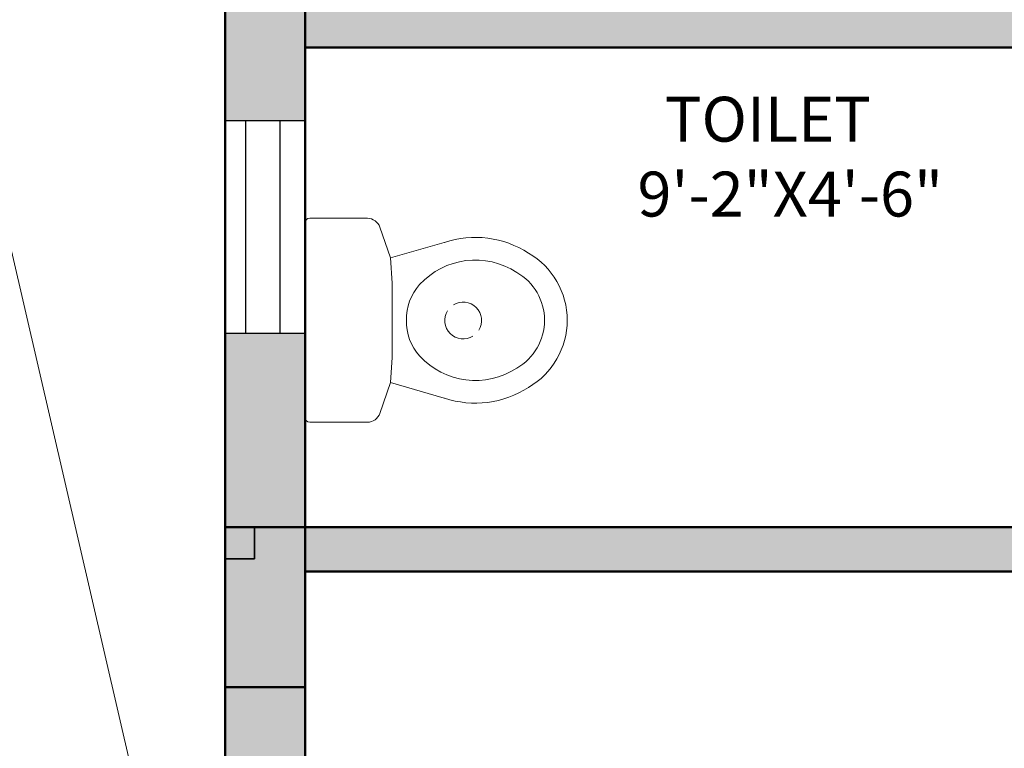
# Model space of a CAD drawing. Units: inches. Extents: x -7 to 1228, y -146 to 1091.
# Tile 70 of 88: x 611 to 722, y 703 to 785. Entities that reach past the tile are written whole.
import ezdxf

# ---------------------------------------------------------------- set-up
doc = ezdxf.new("R2010")
doc.units = ezdxf.units.IN
for name, color, linetype, lineweight in [('A-AREA-IDEN', 7, 'Continuous', 18), ('A-COLS', 6, 'Continuous', 35), ('A-FLOR-FIXT', 8, 'Continuous', 18), ('A-FLOR-VOID', 7, 'Continuous', 18), ('A-GLAZ', 175, 'Continuous', 25), ('A-WALL', 7, 'Continuous', 50), ('A-WALL-PATT', 251, 'Continuous', 13)]:
    doc.layers.add(name, color=color, linetype=linetype, lineweight=lineweight)
doc.styles.get("Standard").update_dxf_attribs({"font": 'arial.ttf'})

# ---------------------------------------------------------------- blocks, each defined once
blk = doc.blocks.new('A$C7B5C7CD4')
at = {"ltscale": 20}
for p, q in [((0, 0.614), (0, 0.4765)), ((0.243, 0.625), (0.011, 0.625)), ((0.243, 0.625), (0.475, 0.625)), ((0.486, 0.614), (0.486, 0.4765)), ((0.0212, 0.4467), (0.0946, 0.4214)), ((0.4648, 0.4467), (0.3914, 0.4214)), ((0.0946, 0.4214), (0.0576, 0.293)), ((0.0946, 0.4214), (0.1544, 0.4173)), ((0.3316, 0.4173), (0.1544, 0.4173)), ((0.3914, 0.4214), (0.3316, 0.4173)), ((0.3914, 0.4214), (0.4284, 0.293))]:
    blk.add_line(p, q, dxfattribs=at)
for centre, radius, start, end in [((0.011, 0.614), 0.011, 90, 180), ((0.475, 0.614), 0.011, 0, 90), ((0.0315, 0.4765), 0.0315, 180, 251), ((0.4545, 0.4765), 0.0315, 289, 0), ((0.24, 0.2602), 0.123, 88.6158, 131.7414), ((0.246, 0.2602), 0.123, 48.2586, 91.3842), ((0.2796, 0.219), 0.18, 132.4207, 213.289), ((0.2064, 0.219), 0.18, 326.711, 47.5793), ((0.2796, 0.219), 0.234, 161.5846, 212.8753), ((0.2064, 0.219), 0.234, 327.1247, 18.4154), ((0.243, 0.185), 0.131, 209.6292, 270), ((0.243, 0.185), 0.131, 270, 330.3708), ((0.243, 0.185), 0.185, 210.1745, 270), ((0.243, 0.185), 0.185, 270, 329.8255)]:
    blk.add_arc(centre, radius, start, end, dxfattribs=at)
for start, end in [(58.1785, 211.8215), (238.1785, 31.8215)]:
    blk.add_arc((0.2426, 0.2481), 0.0439, start, end)
blk = doc.blocks.new('WIN-24')
for p, q in [((0, 0), (0, 24)), ((0, 24), (9, 24)), ((2.34, 0), (2.34, 24)), ((2.34, 24), (6.14, 24)), ((6.14, 24), (6.14, 0)), ((9, 24), (9, 0)), ((9, 0), (0, 0))]:
    blk.add_line(p, q)

msp = doc.modelspace()

# ---------------------------------------------------------------- hatches: boundary and pattern name
at = {"layer": 'A-COLS'}
h = msp.add_hatch(color=256, dxfattribs=at)
h.dxf.hatch_style = 1
h.paths.add_polyline_path([(634, 710), (643, 710), (643, 728), (637.29, 728), (637.29, 724.45), (634, 724.45)])
h = msp.add_hatch(color=256, dxfattribs=at)
h.dxf.hatch_style = 1
h.paths.add_polyline_path([(637.29, 724.45), (637.29, 728), (634, 728), (634, 724.45)])
at = {"layer": 'A-WALL-PATT'}
h = msp.add_hatch(color=256, dxfattribs=at)
h.dxf.hatch_style = 1
h.paths.add_polyline_path([(69, 568), (60, 568), (60, 493), (63.29, 493), (69, 493)])
h.paths.add_polyline_path([(69, 662.41), (60, 662.41), (60, 586), (69, 586)], flags=17)
h.paths.add_polyline_path([(69, 723), (184, 723), (184, 734), (179, 734), (179, 728), (69, 728), (69, 741.62), (60, 741.62), (60, 698.41), (69, 698.41)], flags=17)
h.paths.add_polyline_path([(69, 782), (231, 782), (231, 728), (231, 723), (231, 586), (236, 586), (236, 787), (69, 787), (69, 800.13), (60, 800.13), (60, 765.62), (69, 765.62)])
h.paths.add_polyline_path([(184, 842), (189, 842), (189, 848), (173, 848), (173, 842), (179, 842), (179, 787), (184, 787)])
h.paths.add_polyline_path([(118.22, 69), (69, 69), (69, 60), (118.22, 60)])
h.paths.add_polyline_path([(227, 69), (154.22, 69), (154.22, 60), (227, 60)])
h.paths.add_polyline_path([(236, 60), (232.71, 60), (227, 60), (227, 36), (236, 36)])
h.paths.add_polyline_path([(389, 60), (380, 60), (380, 36), (389, 36)])
h.paths.add_polyline_path([(384, 181), (380, 181), (380, 115), (380, 78), (384, 78)])
h.paths.add_polyline_path([(380, 115), (334.55, 115), (334.55, 109), (380, 109)])
h.paths.add_polyline_path([(274.55, 115), (236, 115), (236, 201), (232.71, 201), (231, 201), (231, 78), (236, 78), (236, 109), (274.55, 109)])
h.paths.add_polyline_path([(69, 123), (60, 123), (60, 78), (69, 78)])
h.paths.add_polyline_path([(69, 201), (60, 201), (60, 159), (69, 159)])
h.paths.add_polyline_path([(143, 219), (69, 219), (69, 213), (143, 213)], flags=17)
h.paths.add_polyline_path([(189, 219), (184, 219), (184, 274), (231, 274), (231, 219), (236, 219), (236, 279), (184, 279), (184, 297), (179, 297), (179, 279), (69, 279), (69, 290.91), (60, 290.91), (60, 262.18), (69, 262.18), (69, 274), (179, 274), (179, 219), (173, 219), (173, 213), (189, 213)])
h.paths.add_polyline_path([(69, 238.18), (60, 238.18), (60, 219), (69, 219)], flags=17)
h.paths.add_polyline_path([(69, 333), (60, 333), (60, 314.91), (69, 314.91), (69, 316.96)])
h.paths.add_polyline_path([(190, 338), (184, 338), (69, 338), (69, 333), (179, 333), (179, 327), (184, 327), (184, 333.02), (190, 333.05)])
h.paths.add_polyline_path([(69, 386.81), (60, 386.81), (60, 351), (69, 351)])
h.paths.add_polyline_path([(69, 475), (60, 475), (60, 422.81), (69, 422.81)])
h.paths.add_polyline_path([(236, 475), (231, 475), (231, 351.24), (236, 351.24)])
h.paths.add_polyline_path([(384, 475), (380, 475), (380, 362), (384, 362)])
h.paths.add_polyline_path([(547, 307), (439, 307), (439, 356), (445, 356), (445, 362), (433, 362), (433, 307), (380, 307), (380, 244), (380, 241), (384, 241), (384, 301), (433, 301), (433, 277), (439, 277), (439, 301), (547, 301)])
h.paths.add_polyline_path([(547, 241), (439, 241), (439, 247), (433, 247), (433, 235), (547, 235)])
h.paths.add_polyline_path([(450, 69), (440.29, 69), (424.89, 69), (389, 69), (389, 60), (450, 60)])
h.paths.add_polyline_path([(547, 69), (486, 69), (486, 60), (547, 60)])
h.paths.add_polyline_path([(556, 148.27), (547, 148.27), (547, 78), (556, 78)])
h.paths.add_polyline_path([(556, 223), (547, 223), (547, 195), (547, 184.27), (556, 184.27)])
h.paths.add_polyline_path([(556, 311.19), (547, 311.19), (547, 273.08), (556, 273.08)])
h.paths.add_polyline_path([(556, 344), (552.71, 344), (547, 344), (547, 335.19), (556, 335.19)])
h.paths.add_polyline_path([(556, 249.08), (547, 249.08), (547, 241), (556, 241)])
h.paths.add_polyline_path([(547, 362), (475, 362), (475, 356), (547, 356)], flags=0)
h.paths.add_polyline_path([(556, 399.62), (547, 399.62), (547, 362), (556, 362)])
h.paths.add_polyline_path([(556, 475), (547, 475), (547, 435.62), (556, 435.62)])
h.paths.add_polyline_path([(547, 493), (389, 493), (389, 487), (547, 487)])
h.paths.add_polyline_path([(380, 493), (278, 493), (278, 487), (380, 487)])
h.paths.add_polyline_path([(227, 493), (69, 493), (69, 487), (227, 487)])
h.paths.add_polyline_path([(643, 122.44), (634, 122.44), (634, 78), (643, 78)])
h.paths.add_polyline_path([(702.5, 69), (692.79, 69), (677.39, 69), (643, 69), (643, 60), (702.5, 60)])
h.paths.add_polyline_path([(798, 69), (738.5, 69), (738.5, 60), (798, 60)])
h.paths.add_polyline_path([(807, 60), (803.71, 60), (798, 60), (798, 36), (807, 36)])
h.paths.add_polyline_path([(807, 109), (846.75, 109), (846.75, 115), (807, 115), (807, 159), (802, 159), (802, 78), (807, 78)])
h.paths.add_polyline_path([(807, 201), (802, 201), (802, 195), (807, 195)])
h.paths.add_polyline_path([(643, 201), (634, 201), (634, 158.44), (643, 158.44)])
h.paths.add_polyline_path([(756, 225), (751, 225), (751, 219), (643, 219), (643, 213), (756, 213)])
h.paths.add_polyline_path([(643, 240.85), (634, 240.85), (634, 219), (643, 219)])
h.paths.add_polyline_path([(643, 274), (643, 288.63), (634, 288.63), (634, 264.85), (643, 264.85)])
h.paths.add_polyline_path([(802, 279), (756, 279), (756, 297), (751, 297), (751, 279), (643, 279), (643, 274), (751, 274), (751, 255), (756, 255), (756, 274), (802, 274)])
h.paths.add_polyline_path([(807, 333), (803.71, 333), (802, 333), (802, 279), (802, 274), (802, 219), (807, 219)])
h.paths.add_polyline_path([(956, 182), (951, 182), (951, 115), (906.75, 115), (906.75, 109), (951, 109), (951, 78), (956, 78)])
h.paths.add_polyline_path([(960, 60), (951, 60), (951, 36), (960, 36)])
h.paths.add_polyline_path([(1021, 69), (1005.78, 69), (960, 69), (960, 60), (1021, 60)])
h.paths.add_polyline_path([(956, 224), (951, 224), (951, 218), (956, 218)])
h.paths.add_polyline_path([(956, 302), (1004, 302), (1004, 278), (1010, 278), (1010, 302), (1118, 302), (1118, 290.81), (1127, 290.81), (1127, 326.97), (1118, 326.97), (1118, 320.97), (1118, 307), (1010, 307), (1010, 356), (1016, 356), (1016, 362), (1004, 362), (1004, 307), (951, 307), (951, 244), (951, 242), (954.29, 242), (956, 242)])
h.paths.add_polyline_path([(643, 333), (634, 333), (634, 312.63), (643, 312.63), (643, 316.96)])
h.paths.add_polyline_path([(756, 338), (643, 338), (643, 333), (751, 333), (751, 327), (756, 327)])
h.paths.add_polyline_path([(643, 388), (634, 388), (634, 351), (643, 351)])
h.paths.add_polyline_path([(807, 357), (802, 357), (802, 351), (807, 351)])
h.paths.add_polyline_path([(807, 475), (802, 475), (802, 393), (807, 393)])
h.paths.add_polyline_path([(643, 475), (634, 475), (634, 424), (643, 424)])
h.paths.add_polyline_path([(798, 493), (643, 493), (643, 487), (798, 487)])
h.paths.add_polyline_path([(634, 493), (556, 493), (556, 487), (634, 487)])
h.paths.add_polyline_path([(813, 493), (807, 493), (807, 487), (813, 487)])
h.paths.add_polyline_path([(951, 493), (849, 493), (849, 487), (951, 487)])
h.paths.add_polyline_path([(956, 484), (951, 484), (951, 374), (956, 374)])
h.paths.add_polyline_path([(1109, 493), (969, 493), (969, 487), (1109, 487)])
h.paths.add_polyline_path([(1127, 484), (1118, 484), (1118, 450.64), (1127, 450.64)])
h.paths.add_polyline_path([(1127, 414.64), (1118, 414.64), (1118, 365), (1127, 365)])
h.paths.add_polyline_path([(1109, 362), (1046, 362), (1046, 356), (1109, 356)], flags=17)
h.paths.add_polyline_path([(1127, 356), (1123.45, 356), (1118, 356), (1118, 350.97), (1127, 350.97)], flags=0)
h.paths.add_polyline_path([(1127, 266.81), (1118, 266.81), (1118, 262.36), (1118, 242), (1127, 242)], flags=17)
h.paths.add_polyline_path([(1118, 242), (1010, 242), (1010, 248), (1004, 248), (1004, 237), (1118, 237)])
h.paths.add_polyline_path([(1127, 224), (1118, 224), (1118, 170), (1127, 170)])
h.paths.add_polyline_path([(1127, 134), (1118, 134), (1118, 78), (1127, 78)])
h.paths.add_polyline_path([(1118, 69), (1057, 69), (1057, 60), (1118, 60)])
h.paths.add_polyline_path([(227, 571.55), (227, 574), (69, 574), (69, 568), (227, 568)])
h.paths.add_polyline_path([(380, 571.55), (380, 574), (278, 574), (278, 568), (380, 568)])
h.paths.add_polyline_path([(242, 574), (236, 574), (236, 568), (242, 568)])
h.paths.add_polyline_path([(547, 571.55), (547, 574), (389, 574), (389, 568), (547, 568)])
h.paths.add_polyline_path([(384, 733), (380, 733), (380, 586), (384, 586)])
h.paths.add_polyline_path([(556, 646), (634, 646), (634, 655), (547, 655), (547, 586), (556, 586)])
h.paths.add_polyline_path([(634, 574), (556, 574), (556, 568), (634, 568)])
h.paths.add_polyline_path([(643, 655), (634, 655), (634, 586), (643, 586)])
h.paths.add_polyline_path([(798, 574), (643, 574), (643, 568), (798, 568)])
h.paths.add_polyline_path([(643, 663.85), (634, 663.85), (634, 655), (643, 655)])
h.paths.add_polyline_path([(556, 676.97), (547, 676.97), (547, 655), (556, 655)])
h.paths.add_polyline_path([(556, 733), (547, 733), (547, 712.97), (556, 712.97)])
h.paths.add_polyline_path([(643, 710), (634, 710), (634, 699.85), (643, 699.85)])
h.paths.add_polyline_path([(807, 668), (802, 668), (802, 586), (807, 586)])
h.paths.add_polyline_path([(951, 574), (849, 574), (849, 568), (951, 568)])
h.paths.add_polyline_path([(956, 691), (951, 691), (951, 577), (956, 577)])
h.paths.add_polyline_path([(1109, 574), (969, 574), (969, 568), (1109, 568)])
h.paths.add_polyline_path([(1127, 643.4), (1118, 643.4), (1118, 577), (1127, 577)])
h.paths.add_polyline_path([(1127, 568), (1123.45, 568), (1118, 568), (1118, 493), (1127, 493)])
h.paths.add_polyline_path([(1127, 733), (1118, 733), (1118, 679.4), (1127, 679.4)])
h.paths.add_polyline_path([(1127, 777.35), (1118, 777.35), (1118, 770.04), (1118, 751), (1127, 751)], flags=17)
h.paths.add_polyline_path([(1118, 751), (1010, 751), (1010, 757), (1004, 757), (1004, 745), (1118, 745)])
h.paths.add_polyline_path([(956, 811), (1004, 811), (1004, 787), (1010, 787), (1010, 811), (1017.87, 811), (1017.87, 811.63, -0.414214), (1018.25, 812), (1031.98, 812, -0.414214), (1032.35, 811.63), (1032.35, 811), (1118, 811), (1118, 801.35), (1127, 801.35), (1127, 834.69), (1118, 834.69), (1118, 830.24), (1118, 817), (1010, 817), (1010, 866), (1016, 866), (1016, 872), (1004, 872), (1004, 817), (956, 817), (956, 866), (951, 866), (951, 751), (954.29, 751), (956, 751)])
h.paths.add_polyline_path([(1118, 872), (1046, 872), (1046, 866), (1118, 866)], flags=17)
h.paths.add_polyline_path([(1127, 924.71), (1118, 924.71), (1118, 884), (1127, 884)])
h.paths.add_polyline_path([(1127, 866), (1123.71, 866), (1118, 866), (1118, 858.69), (1127, 858.69)], flags=17)
h.paths.add_polyline_path([(956, 983), (951, 983), (951, 952), (807, 952), (807, 983), (802, 983), (802, 902), (807, 902), (807, 946), (951, 946), (951, 884), (956, 884)])
h.paths.add_polyline_path([(807, 842), (802, 842), (802, 787), (756, 787), (756, 806), (751, 806), (751, 787), (643, 787), (643, 782), (751, 782), (751, 764), (756, 764), (756, 782), (802, 782), (802, 728), (807, 728)])
h.paths.add_polyline_path([(756, 848), (643, 848), (643, 842), (751, 842), (751, 836), (756, 836)])
h.paths.add_polyline_path([(756, 734), (751, 734), (751, 728), (643, 728), (643, 723), (756, 723)])
h.paths.add_polyline_path([(643, 749.79), (634, 749.79), (634, 728), (637.29, 728), (643, 728)])
h.paths.add_polyline_path([(643, 805.41), (634, 805.41), (634, 773.79), (643, 773.79)])
h.paths.add_polyline_path([(643, 896.66), (634, 896.66), (634, 860), (637.29, 860), (643, 860)])
h.paths.add_polyline_path([(643, 842), (634, 842), (634, 829.41), (643, 829.41)])
h.paths.add_polyline_path([(643, 983), (634, 983), (634, 932.66), (643, 932.66)])
h.paths.add_polyline_path([(1127, 983), (1118, 983), (1118, 960.71), (1127, 960.71)])
h.paths.add_polyline_path([(1118, 1001), (1077.53, 1001), (1077.53, 992), (1118, 992)])
h.paths.add_polyline_path([(1041.53, 1001), (960, 1001), (960, 992), (1041.53, 992)])
h.paths.add_polyline_path([(960, 1025), (951, 1025), (951, 1001), (954.29, 1001), (960, 1001)])
h.paths.add_polyline_path([(807, 1025), (798, 1025), (798, 1001), (807, 1001)])
h.paths.add_polyline_path([(798, 1001), (738.5, 1001), (738.5, 992), (798, 992)])
h.paths.add_polyline_path([(702.5, 1001), (643, 1001), (643, 992), (702.5, 992)])
h.paths.add_polyline_path([(547, 1001), (499.11, 1001), (499.11, 992), (547, 992)])
h.paths.add_polyline_path([(463.11, 1001), (389, 1001), (389, 992), (463.11, 992)])
h.paths.add_polyline_path([(389, 1025), (380, 1025), (380, 1022), (380, 1001), (383.29, 1001), (389, 1001)])
h.paths.add_polyline_path([(236, 1025), (227, 1025), (227, 1001), (236, 1001)])
h.paths.add_polyline_path([(236, 983), (231, 983), (231, 860), (236, 860)])
h.paths.add_polyline_path([(274.55, 952), (236, 952), (236, 946), (274.55, 946)])
h.paths.add_polyline_path([(380, 952), (334.55, 952), (334.55, 946), (380, 946)])
h.paths.add_polyline_path([(384, 983), (380, 983), (380, 884), (383.29, 884), (384, 884)])
h.paths.add_polyline_path([(227, 1001), (155.01, 1001), (155.01, 992), (162.87, 992), (227, 992)])
h.paths.add_polyline_path([(119.01, 1001), (69, 1001), (69, 992), (119.01, 992)])
h.paths.add_polyline_path([(69, 983), (60, 983), (60, 922.99), (69, 922.99)])
h.paths.add_polyline_path([(69, 886.99), (60, 886.99), (60, 860), (63.29, 860), (69, 860)])
h.paths.add_polyline_path([(143, 848), (69, 848), (69, 842), (143, 842)])

# ---------------------------------------------------------------- linework, layer by layer
at = {"layer": 'A-COLS'}
msp.add_lwpolyline([(634, 728), (637.29, 728), (637.29, 724.45), (634, 724.45)], close=True, dxfattribs=at)
at = {"layer": 'A-FLOR-VOID'}
msp.add_line((556, 992), (634, 655), dxfattribs=at)
at = {"layer": 'A-WALL'}
for p, q in [((634, 1001), (634, 655)), ((634, 568), (634, 1001)), ((643, 568), (643, 1001)), ((643, 782), (643, 728)), ((751, 782), (643, 782)), ((634, 728), (643, 728)), ((634, 710), (634, 728)), ((751, 728), (643, 728)), ((643, 728), (643, 710)), ((643, 723), (643, 568)), ((756, 723), (643, 723)), ((643, 710), (643, 716)), ((643, 710), (634, 710))]:
    msp.add_line(p, q, dxfattribs=at)

# ---------------------------------------------------------------- block references
at = {"layer": 'A-FLOR-FIXT', "xscale": 47.26153857112405, "yscale": 47.26153857112405, "zscale": 47.26153857112405, "rotation": 90}
msp.add_blockref('A$C7B5C7CD4', (672.54, 739.81), dxfattribs=at)
at = {"layer": 'A-GLAZ'}
msp.add_blockref('WIN-24', (634, 749.79), dxfattribs=at)

# ---------------------------------------------------------------- texts
at = {"layer": 'A-AREA-IDEN', "insert": (680.46, 776.46), "char_height": 5.0568, "attachment_point": 1}
msp.add_mtext_dynamic_manual_height_columns('  TOILET\\P9\'-2"X4\'-6"', width=137.2821, gutter_width=25.28, heights=[0], dxfattribs=at)

doc.saveas('drawing.dxf')
